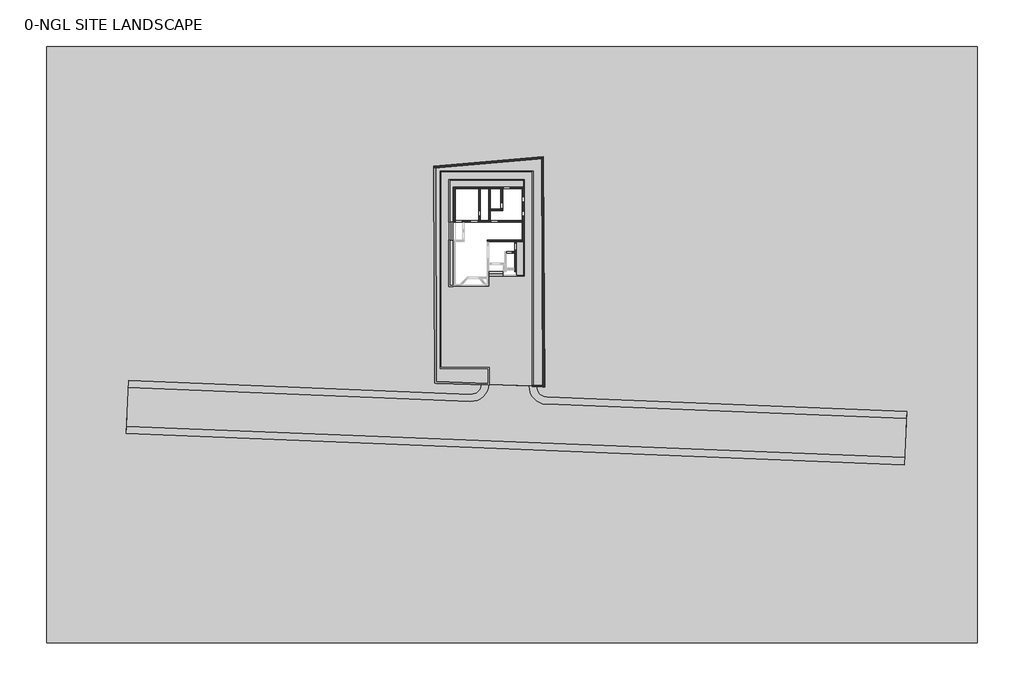
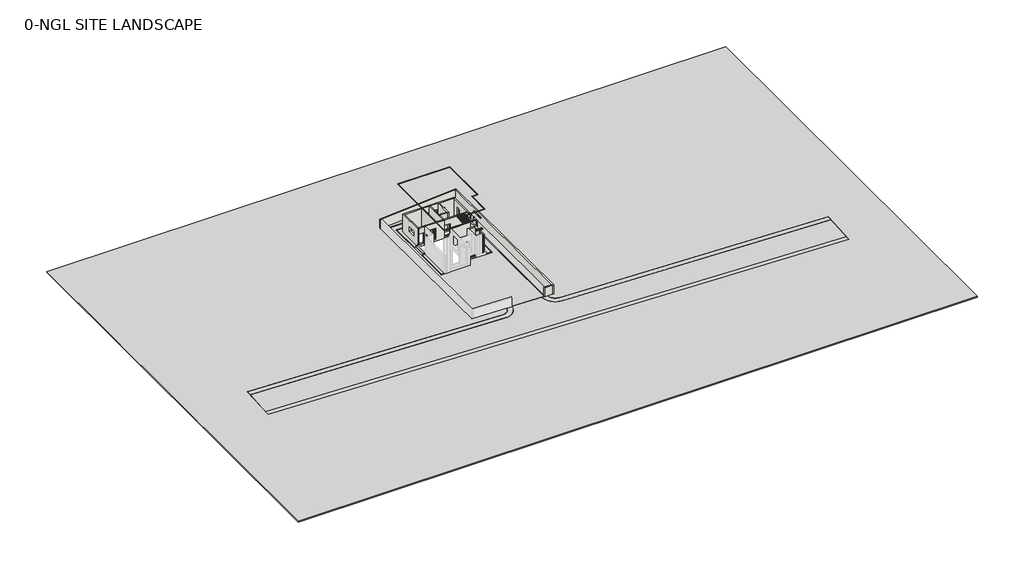
# One storey, part 2 of 2: 21 walls, 2 stair flights, 1 furniture element, 1 proxy.
"""IFC4 building model written with IfcOpenShell, lengths in millimetres."""

from ifc_helpers import new_model, si_unit, frame, origin, origin_with_axes, place, context, project, spatial, polyline, outline, extrude, faceted_brep, transform, mapped, element, save
from components import site_road_site_road_cda8f1bc, casework_1_casework_1_205f5306

model = new_model("IFC4")

# Units and contexts
model_context = context("Model", 3, world=origin())
ifc_project = project(units=[si_unit("LENGTHUNIT", "METRE", prefix="MILLI")], contexts=[model_context])

# Site, building, storey
site = spatial("IfcSite", under=ifc_project)
building = spatial("IfcBuilding", under=site)
storey = spatial("IfcBuildingStorey", under=building, Name="0-NGL SITE LANDSCAPE", Elevation=0.0)

# Proxy
placement = place(None, origin())
site_road_site_road_shape = site_road_site_road_cda8f1bc(model_context)
element("IfcBuildingElementProxy", 1, Name="SITE ROAD : SITE ROAD", ObjectType="SITE ROAD : SITE ROAD", at=placement, inside=storey, context=model_context, shape_type="MappedRepresentation", body=[
    mapped(site_road_site_road_shape, transform((0.0, 0.0, 0.0), x_axis=(1.0, 0.0, 0.0), y_axis=(0.0, 1.0, 0.0), z_axis=(0.0, 0.0, 1.0))),
])

# Furniture
casework_1_casework_1_shape = casework_1_casework_1_205f5306(model_context)
element("IfcFurniture", 2, ObjectType="Casework 1 : Casework 1", at=placement, inside=storey, context=model_context, shape_type="MappedRepresentation", body=[
    mapped(casework_1_casework_1_shape, transform((0.0, 0.0, 0.0), x_axis=(1.0, 0.0, 0.0), y_axis=(0.0, 1.0, 0.0), z_axis=(0.0, 0.0, 1.0))),
])

# Stair flights
element("IfcStairFlight", 3, ObjectType="150mm Depth", at=placement, inside=storey, context=model_context, shape_type="Brep", body=[
    faceted_brep([(-10608.8712297, -1317.0014262, 150.0), (-10908.8712297, -1317.0014262, 150.0), (-10908.8712297, -3817.0014262, 150.0), (-10608.8712297, -3817.0014262, 150.0), (-10608.8712297, -1317.0014262, 0.0), (-10908.8712297, -1317.0014262, 0.0), (-10908.8712297, -3817.0014262, 0.0), (-10608.8712297, -3817.0014262, 0.0), (-10308.8712297, -1317.0014262, 300.0), (-10608.8712297, -1317.0014262, 300.0), (-10608.8712297, -3817.0014262, 300.0), (-10308.8712297, -3817.0014262, 300.0), (-10308.8712297, -1317.0014262, 132.2949017), (-10573.461033, -1317.0014262, 0.0), (-10573.461033, -3817.0014262, 0.0), (-10308.8712297, -3817.0014262, 132.2949017)], [[[0, 1, 2, 3]], [[1, 0, 4, 5]], [[2, 1, 5, 6]], [[3, 2, 6, 7]], [[8, 9, 10, 11]], [[4, 0, 9, 8, 12, 13]], [[0, 3, 10, 9]], [[3, 7, 14, 15, 11, 10]], [[8, 11, 15, 12]], [[5, 4, 13, 14, 7, 6]], [[14, 13, 12, 15]]]),
])
element("IfcStairFlight", 4, ObjectType="150mm Depth", at=placement, inside=storey, context=model_context, shape_type="Brep", body=[
    faceted_brep([(-5348.8712297, -8577.0014262, 150.0), (-5348.8712297, -8877.0014262, 150.0), (-3308.8712297, -8877.0014262, 150.0), (-3308.8712297, -8577.0014262, 150.0), (-5348.8712297, -8577.0014262, 0.0), (-5348.8712297, -8877.0014262, 0.0), (-3308.8712297, -8877.0014262, 0.0), (-3308.8712297, -8577.0014262, 0.0), (-5348.8712297, -8277.0014262, 300.0), (-5348.8712297, -8577.0014262, 300.0), (-3308.8712297, -8577.0014262, 300.0), (-3308.8712297, -8277.0014262, 300.0), (-5348.8712297, -8277.0014262, 132.2949017), (-5348.8712297, -8541.5912295, 0.0), (-3308.8712297, -8541.5912295, 0.0), (-3308.8712297, -8277.0014262, 132.2949017)], [[[0, 1, 2, 3]], [[1, 0, 4, 5]], [[2, 1, 5, 6]], [[3, 2, 6, 7]], [[8, 9, 10, 11]], [[4, 0, 9, 8, 12, 13]], [[0, 3, 10, 9]], [[3, 7, 14, 15, 11, 10]], [[8, 11, 15, 12]], [[5, 4, 13, 14, 7, 6]], [[14, 13, 12, 15]]]),
])

# Walls
element("IfcWall", 5, ObjectType="100", at=placement, inside=storey, context=model_context, shape_type="Brep", body=[
    faceted_brep([(-308.8712297, -8927.0014262, 0.0), (-308.8712297, -4047.0014262, 0.0), (-308.8712297, -4047.0014262, 150.0), (-308.8712297, -8927.0014262, 150.0), (-408.8712297, -8927.0014262, 0.0), (-408.8712297, -8927.0014262, 150.0), (-408.8712297, -8827.0014262, 150.0), (-408.8712297, -4047.0014262, 150.0), (-408.8712297, -4047.0014262, 0.0), (-408.8712297, -8827.0014262, 0.0), (-358.8712297, -4047.0014262, 0.0)], [[[0, 1, 2, 3]], [[4, 5, 6, 7, 8, 9]], [[1, 0, 4, 9, 8, 10]], [[3, 2, 7, 6, 5]], [[2, 1, 10, 8, 7]], [[0, 3, 5, 4]]]),
])
element("IfcWall", 6, ObjectType="100", at=placement, inside=storey, context=model_context, shape_type="Brep", body=[
    faceted_brep([(-10858.8712297, -1317.0014262, 0.0), (-10858.8712297, 4592.9985738, 0.0), (-10858.8712297, 4692.9985738, 0.0), (-10858.8712297, 4692.9985738, 150.0), (-10858.8712297, 4592.9985738, 150.0), (-10858.8712297, -1317.0014262, 150.0), (-10958.8712297, -1317.0014262, 0.0), (-10958.8712297, -1317.0014262, 150.0), (-10958.8712297, 4692.9985738, 150.0), (-10958.8712297, 4692.9985738, 0.0)], [[[0, 1, 2, 3, 4, 5]], [[6, 7, 8, 9]], [[2, 1, 0, 6, 9]], [[5, 4, 3, 8, 7]], [[0, 5, 7, 6]], [[3, 2, 9, 8]]]),
])
element("IfcWall", 7, ObjectType="100", at=placement, inside=storey, context=model_context, shape_type="Brep", body=[
    faceted_brep([(891.1287703, -24267.7575352, 0.0), (891.1287703, 5892.9985738, 0.0), (891.1287703, 5892.9985738, 150.0), (891.1287703, -24267.7575352, 150.0), (791.1287703, -24264.1774027, 0.0), (791.1287703, -24264.1774027, 150.0), (791.1287703, 5792.9985738, 150.0), (791.1287703, 5892.9985738, 150.0), (791.1287703, 5892.9985738, 0.0), (791.1287703, 5792.9985738, 0.0)], [[[0, 1, 2, 3]], [[4, 5, 6, 7, 8, 9]], [[1, 0, 4, 9, 8]], [[3, 2, 7, 6, 5]], [[0, 3, 5, 4]], [[2, 1, 8, 7]]]),
])
element("IfcWall", 8, ObjectType="100", at=placement, inside=storey, context=model_context, shape_type="Brep", body=[
    faceted_brep([(-10858.8712297, 4592.9985738, 0.0), (-408.8712297, 4592.9985738, 0.0), (-308.8712297, 4592.9985738, 0.0), (-308.8712297, 4592.9985738, 150.0), (-408.8712297, 4592.9985738, 150.0), (-10858.8712297, 4592.9985738, 150.0), (-10858.8712297, 4692.9985738, 0.0), (-10858.8712297, 4692.9985738, 150.0), (-308.8712297, 4692.9985738, 150.0), (-308.8712297, 4692.9985738, 0.0)], [[[0, 1, 2, 3, 4, 5]], [[6, 7, 8, 9]], [[2, 1, 0, 6, 9]], [[5, 4, 3, 8, 7]], [[3, 2, 9, 8]], [[0, 5, 7, 6]]]),
])
element("IfcWall", 9, ObjectType="100", at=placement, inside=storey, context=model_context, shape_type="Brep", body=[
    faceted_brep([(-308.8712297, 3642.9985738, 0.0), (-308.8712297, 4592.9985738, 0.0), (-308.8712297, 4592.9985738, 150.0), (-308.8712297, 3642.9985738, 150.0), (-408.8712297, 3642.9985738, 0.0), (-408.8712297, 3642.9985738, 150.0), (-408.8712297, 4592.9985738, 150.0), (-408.8712297, 4592.9985738, 0.0), (-358.8712297, 3642.9985738, 0.0)], [[[0, 1, 2, 3]], [[4, 5, 6, 7]], [[1, 0, 8, 4, 7]], [[3, 2, 6, 5]], [[2, 1, 7, 6]], [[0, 3, 5, 4, 8]]]),
])
element("IfcWall", 10, ObjectType="100", at=placement, inside=storey, context=model_context, shape_type="SweptSolid", body=[
    extrude(outline(polyline([(791.1287703, 5792.9985738), (-12058.8712297, 5792.9985738), (-12058.8712297, 5892.9985738), (791.1287703, 5892.9985738), (791.1287703, 5792.9985738)])), origin_with_axes(), (0.0, 0.0, 1.0), 150.0),
])
element("IfcWall", 11, ObjectType="230", at=placement, inside=storey, context=model_context, shape_type="Brep", body=[
    faceted_brep([(-588.8712297, -3817.0014262, 3750.0), (-588.8712297, -3817.0014262, 0.0), (-5578.8712297, -3817.0014262, 0.0), (-5578.8712297, -3817.0014262, 3750.0), (-588.8712297, -4047.0014262, 0.0), (-588.8712297, -4047.0014262, 3750.0), (-1448.8712297, -4047.0014262, 3750.0), (-1678.8712297, -4047.0014262, 3750.0), (-5348.8712297, -4047.0014262, 3750.0), (-5578.8712297, -4047.0014262, 3750.0), (-5578.8712297, -4047.0014262, 0.0), (-5348.8712297, -4047.0014262, 0.0), (-1678.8712297, -4047.0014262, 0.0), (-1448.8712297, -4047.0014262, 0.0)], [[[0, 1, 2, 3]], [[4, 5, 6, 7, 8, 9, 10, 11, 12, 13]], [[2, 1, 4, 13, 12, 11, 10]], [[0, 3, 9, 8, 7, 6, 5]], [[3, 2, 10, 9]], [[0, 5, 4, 1]]]),
])
element("IfcWall", 12, ObjectType="230", at=placement, inside=storey, context=model_context, shape_type="Brep", body=[
    faceted_brep([(-10308.8712297, 3642.9985738, 0.0), (-10308.8712297, -1202.0014262, 0.0), (-10308.8712297, -1202.0014262, 450.0), (-10308.8712297, -1317.0014262, 450.0), (-10308.8712297, -1317.0014262, 3750.0), (-10308.8712297, 3642.9985738, 3750.0), (-10308.8712297, -82.0014262, 1650.0), (-10308.8712297, 1417.9985738, 1650.0), (-10308.8712297, 1417.9985738, 2550.0), (-10308.8712297, -82.0014262, 2550.0), (-10078.8712297, 3642.9985738, 0.0), (-10078.8712297, 3642.9985738, 3750.0), (-10078.8712297, 3412.9985738, 3750.0), (-10078.8712297, -1087.0014262, 3750.0), (-10078.8712297, -1317.0014262, 3750.0), (-10078.8712297, -1317.0014262, 450.0), (-10078.8712297, -1202.0014262, 450.0), (-10078.8712297, -1202.0014262, 0.0), (-10078.8712297, -1087.0014262, 0.0), (-10078.8712297, 3412.9985738, 0.0), (-10078.8712297, -82.0014262, 1650.0), (-10078.8712297, -82.0014262, 2550.0), (-10078.8712297, 1417.9985738, 2550.0), (-10078.8712297, 1417.9985738, 1650.0)], [[[0, 1, 2, 3, 4, 5], [6, 7, 8, 9]], [[10, 11, 12, 13, 14, 15, 16, 17, 18, 19], [20, 21, 22, 23]], [[1, 0, 10, 19, 18, 17]], [[5, 4, 14, 13, 12, 11]], [[0, 5, 11, 10]], [[21, 20, 6, 9]], [[22, 21, 9, 8]], [[23, 22, 8, 7]], [[20, 23, 7, 6]], [[2, 1, 17, 16]], [[15, 3, 2, 16]], [[4, 3, 15, 14]]]),
])
element("IfcWall", 13, ObjectType="230", at=placement, inside=storey, context=model_context, shape_type="Brep", body=[
    faceted_brep([(-1448.8712297, -8277.0014262, 0.0), (-1448.8712297, -4047.0014262, 0.0), (-1448.8712297, -4047.0014262, 3750.0), (-1448.8712297, -8277.0014262, 3750.0), (-1448.8712297, -8277.0014262, 500.0), (-1448.8712297, -4239.5014262, 900.0), (-1448.8712297, -5239.5014262, 900.0), (-1448.8712297, -5239.5014262, 2550.0), (-1448.8712297, -4239.5014262, 2550.0), (-1448.8712297, -6482.0014262, 1950.0), (-1448.8712297, -7382.0014262, 1950.0), (-1448.8712297, -7382.0014262, 2550.0), (-1448.8712297, -6482.0014262, 2550.0), (-1678.8712297, -8277.0014262, 0.0), (-1678.8712297, -8277.0014262, 3750.0), (-1678.8712297, -8047.0014262, 3750.0), (-1678.8712297, -7817.0014262, 3750.0), (-1678.8712297, -5662.0014262, 3750.0), (-1678.8712297, -5432.0014262, 3750.0), (-1678.8712297, -4047.0014262, 3750.0), (-1678.8712297, -4047.0014262, 0.0), (-1678.8712297, -5432.0014262, 0.0), (-1678.8712297, -5662.0014262, 0.0), (-1678.8712297, -7817.0014262, 0.0), (-1678.8712297, -8047.0014262, 0.0), (-1678.8712297, -4239.5014262, 900.0), (-1678.8712297, -4239.5014262, 2550.0), (-1678.8712297, -5239.5014262, 2550.0), (-1678.8712297, -5239.5014262, 900.0), (-1678.8712297, -6482.0014262, 1950.0), (-1678.8712297, -6482.0014262, 2550.0), (-1678.8712297, -7382.0014262, 2550.0), (-1678.8712297, -7382.0014262, 1950.0), (-1548.8712297, -8277.0014262, 0.0)], [[[0, 1, 2, 3, 4], [5, 6, 7, 8], [9, 10, 11, 12]], [[13, 14, 15, 16, 17, 18, 19, 20, 21, 22, 23, 24], [25, 26, 27, 28], [29, 30, 31, 32]], [[1, 0, 33, 13, 24, 23, 22, 21, 20]], [[3, 2, 19, 18, 17, 16, 15, 14]], [[0, 4, 3, 14, 13, 33]], [[2, 1, 20, 19]], [[26, 25, 5, 8]], [[27, 26, 8, 7]], [[28, 27, 7, 6]], [[25, 28, 6, 5]], [[30, 29, 9, 12]], [[31, 30, 12, 11]], [[32, 31, 11, 10]], [[29, 32, 10, 9]]]),
])
element("IfcWall", 14, ObjectType="230", at=placement, inside=storey, context=model_context, shape_type="Brep", body=[
    faceted_brep([(-10078.8712297, -1317.0014262, 0.0), (-9008.8712297, -1317.0014262, 0.0), (-8778.8712297, -1317.0014262, 0.0), (-5118.8712297, -1317.0014262, 0.0), (-5118.8712297, -1317.0014262, 3750.0), (-8778.8712297, -1317.0014262, 3750.0), (-9008.8712297, -1317.0014262, 3750.0), (-10078.8712297, -1317.0014262, 3750.0), (-10078.8712297, -1317.0014262, 450.0), (-9068.8712297, -1317.0014262, 450.0), (-10018.8712297, -1317.0014262, 450.0), (-10018.8712297, -1317.0014262, 2575.0), (-9068.8712297, -1317.0014262, 2575.0), (-7916.1212297, -1317.0014262, 2639.5), (-6811.6212297, -1317.0014262, 2639.5), (-6811.6212297, -1317.0014262, 450.0), (-7916.1212297, -1317.0014262, 450.0), (-5118.8712297, -1087.0014262, 0.0), (-5348.8712297, -1087.0014262, 0.0), (-6548.8712297, -1087.0014262, 0.0), (-6778.8712297, -1087.0014262, 0.0), (-10078.8712297, -1087.0014262, 0.0), (-10078.8712297, -1087.0014262, 3750.0), (-6778.8712297, -1087.0014262, 3750.0), (-6548.8712297, -1087.0014262, 3750.0), (-5348.8712297, -1087.0014262, 3750.0), (-5118.8712297, -1087.0014262, 3750.0), (-9068.8712297, -1087.0014262, 450.0), (-9068.8712297, -1087.0014262, 2575.0), (-10018.8712297, -1087.0014262, 2575.0), (-10018.8712297, -1087.0014262, 450.0), (-6811.6212297, -1087.0014262, 2639.5), (-7916.1212297, -1087.0014262, 2639.5), (-7916.1212297, -1087.0014262, 450.0), (-6811.6212297, -1087.0014262, 450.0), (-10078.8712297, -1202.0014262, 0.0), (-6811.6212297, -1107.0014262, 2639.5), (-7916.1212297, -1107.0014262, 2639.5), (-7916.1212297, -1184.0014262, 2639.5), (-6811.6212297, -1184.0014262, 2639.5), (-6811.6212297, -1107.0014262, 450.0), (-6811.6212297, -1184.0014262, 450.0), (-7916.1212297, -1107.0014262, 450.0), (-7931.1212297, -1107.0014262, 450.0), (-7931.1212297, -1184.0014262, 450.0), (-7916.1212297, -1184.0014262, 450.0), (-6796.6212297, -1184.0014262, 450.0), (-6796.6212297, -1107.0014262, 450.0), (-7931.1212297, -1107.0014262, 2654.5), (-6796.6212297, -1107.0014262, 2654.5), (-6796.6212297, -1184.0014262, 2654.5), (-7931.1212297, -1184.0014262, 2654.5)], [[[0, 1, 2, 3, 4, 5, 6, 7, 8], [9, 10, 11, 12], [13, 14, 15, 16]], [[17, 18, 19, 20, 21, 22, 23, 24, 25, 26], [27, 28, 29, 30], [31, 32, 33, 34]], [[3, 2, 1, 0, 35, 21, 20, 19, 18, 17]], [[7, 6, 5, 4, 26, 25, 24, 23, 22]], [[4, 3, 17, 26]], [[7, 22, 21, 35, 0, 8]], [[28, 27, 9, 12]], [[29, 28, 12, 11]], [[30, 29, 11, 10]], [[27, 30, 10, 9]], [[31, 36, 37, 32]], [[13, 38, 39, 14]], [[36, 31, 34, 40]], [[14, 39, 41, 15]], [[40, 34, 33, 42, 43, 44, 45, 16, 15, 41, 46, 47]], [[32, 37, 42, 33]], [[38, 13, 16, 45]], [[48, 49, 50, 51]], [[47, 46, 50, 49]], [[39, 38, 45, 44, 51, 50, 46, 41]], [[44, 43, 48, 51]], [[37, 36, 40, 47, 49, 48, 43, 42]]]),
])
element("IfcWall", 15, ObjectType="230", at=placement, inside=storey, context=model_context, shape_type="Brep", body=[
    faceted_brep([(-5348.8712297, 3412.9985738, 0.0), (-5348.8712297, -1087.0014262, 0.0), (-5348.8712297, -1087.0014262, 3750.0), (-5348.8712297, 3412.9985738, 3750.0), (-5118.8712297, 3412.9985738, 0.0), (-5118.8712297, 3412.9985738, 3750.0), (-5118.8712297, 512.9985738, 3750.0), (-5118.8712297, 282.9985738, 3750.0), (-5118.8712297, -1087.0014262, 3750.0), (-5118.8712297, -1087.0014262, 0.0), (-5118.8712297, 282.9985738, 0.0), (-5118.8712297, 512.9985738, 0.0)], [[[0, 1, 2, 3]], [[4, 5, 6, 7, 8, 9, 10, 11]], [[1, 0, 4, 11, 10, 9]], [[3, 2, 8, 7, 6, 5]], [[0, 3, 5, 4]], [[2, 1, 9, 8]]]),
])
element("IfcWall", 16, ObjectType="230", at=placement, inside=storey, context=model_context, shape_type="Brep", body=[
    faceted_brep([(-10078.8712297, 3412.9985738, 0.0), (-6778.8712297, 3412.9985738, 0.0), (-6548.8712297, 3412.9985738, 0.0), (-5348.8712297, 3412.9985738, 0.0), (-5118.8712297, 3412.9985738, 0.0), (-3618.8712297, 3412.9985738, 0.0), (-3388.8712297, 3412.9985738, 0.0), (-588.8712297, 3412.9985738, 0.0), (-358.8712297, 3412.9985738, 0.0), (-358.8712297, 3412.9985738, 3750.0), (-588.8712297, 3412.9985738, 3750.0), (-3388.8712297, 3412.9985738, 3750.0), (-3618.8712297, 3412.9985738, 3750.0), (-5118.8712297, 3412.9985738, 3750.0), (-5348.8712297, 3412.9985738, 3750.0), (-6548.8712297, 3412.9985738, 3750.0), (-6778.8712297, 3412.9985738, 3750.0), (-10078.8712297, 3412.9985738, 3750.0), (-3303.8712297, 3412.9985738, 900.0), (-3303.8712297, 3412.9985738, 2550.0), (-2303.8712297, 3412.9985738, 2550.0), (-2303.8712297, 3412.9985738, 900.0), (-6398.8712297, 3412.9985738, 1950.0), (-6398.8712297, 3412.9985738, 2550.0), (-5498.8712297, 3412.9985738, 2550.0), (-5498.8712297, 3412.9985738, 1950.0), (-4818.8712297, 3412.9985738, 1950.0), (-4818.8712297, 3412.9985738, 2550.0), (-3918.8712297, 3412.9985738, 2550.0), (-3918.8712297, 3412.9985738, 1950.0), (-10078.8712297, 3642.9985738, 0.0), (-10078.8712297, 3642.9985738, 3750.0), (-358.8712297, 3642.9985738, 3750.0), (-358.8712297, 3642.9985738, 0.0), (-408.8712297, 3642.9985738, 0.0), (-3303.8712297, 3642.9985738, 900.0), (-2303.8712297, 3642.9985738, 900.0), (-2303.8712297, 3642.9985738, 2550.0), (-3303.8712297, 3642.9985738, 2550.0), (-6398.8712297, 3642.9985738, 1950.0), (-5498.8712297, 3642.9985738, 1950.0), (-5498.8712297, 3642.9985738, 2550.0), (-6398.8712297, 3642.9985738, 2550.0), (-4818.8712297, 3642.9985738, 1950.0), (-3918.8712297, 3642.9985738, 1950.0), (-3918.8712297, 3642.9985738, 2550.0), (-4818.8712297, 3642.9985738, 2550.0)], [[[0, 1, 2, 3, 4, 5, 6, 7, 8, 9, 10, 11, 12, 13, 14, 15, 16, 17], [18, 19, 20, 21], [22, 23, 24, 25], [26, 27, 28, 29]], [[30, 31, 32, 33, 34], [35, 36, 37, 38], [39, 40, 41, 42], [43, 44, 45, 46]], [[8, 7, 6, 5, 4, 3, 2, 1, 0, 30, 34, 33]], [[17, 16, 15, 14, 13, 12, 11, 10, 9, 32, 31]], [[0, 17, 31, 30]], [[19, 18, 35, 38]], [[20, 19, 38, 37]], [[21, 20, 37, 36]], [[18, 21, 36, 35]], [[23, 22, 39, 42]], [[24, 23, 42, 41]], [[25, 24, 41, 40]], [[22, 25, 40, 39]], [[27, 26, 43, 46]], [[28, 27, 46, 45]], [[29, 28, 45, 44]], [[26, 29, 44, 43]], [[8, 33, 32, 9]]]),
])
element("IfcWall", 17, ObjectType="230", at=placement, inside=storey, context=model_context, shape_type="SweptSolid", body=[
    extrude(outline(polyline([(3412.9985738, 0.0), (-1087.0014262, 0.0), (-1087.0014262, 3750.0), (3412.9985738, 3750.0), (3412.9985738, 0.0)]), holes=[polyline([(-502.0014262, 450.0), (297.9985738, 450.0), (297.9985738, 2575.0), (-502.0014262, 2575.0), (-502.0014262, 450.0)])]), frame((-6778.8712297, 0.0, 0.0), z_axis=(1.0, 0.0, 0.0), x_axis=(0.0, 1.0, 0.0)), (0.0, 0.0, 1.0), 230.0),
])
element("IfcWall", 18, ObjectType="230", at=placement, inside=storey, context=model_context, shape_type="Brep", body=[
    faceted_brep([(-3618.8712297, 3412.9985738, 0.0), (-3618.8712297, 512.9985738, 0.0), (-3618.8712297, 282.9985738, 0.0), (-3618.8712297, 282.9985738, 3750.0), (-3618.8712297, 512.9985738, 3750.0), (-3618.8712297, 3412.9985738, 3750.0), (-3618.8712297, 597.9985738, 450.0), (-3618.8712297, 1397.9985738, 450.0), (-3618.8712297, 1397.9985738, 2575.0), (-3618.8712297, 597.9985738, 2575.0), (-3388.8712297, 3412.9985738, 0.0), (-3388.8712297, 3412.9985738, 3750.0), (-3388.8712297, 282.9985738, 3750.0), (-3388.8712297, 282.9985738, 0.0), (-3388.8712297, 597.9985738, 450.0), (-3388.8712297, 597.9985738, 2575.0), (-3388.8712297, 1397.9985738, 2575.0), (-3388.8712297, 1397.9985738, 450.0)], [[[0, 1, 2, 3, 4, 5], [6, 7, 8, 9]], [[10, 11, 12, 13], [14, 15, 16, 17]], [[2, 1, 0, 10, 13]], [[5, 4, 3, 12, 11]], [[0, 5, 11, 10]], [[3, 2, 13, 12]], [[15, 14, 6, 9]], [[16, 15, 9, 8]], [[17, 16, 8, 7]], [[14, 17, 7, 6]]]),
])
element("IfcWall", 19, ObjectType="230", at=placement, inside=storey, context=model_context, shape_type="SweptSolid", body=[
    extrude(outline(polyline([(-5118.8712297, 512.9985738), (-3618.8712297, 512.9985738), (-3618.8712297, 282.9985738), (-5118.8712297, 282.9985738), (-5118.8712297, 512.9985738)])), origin_with_axes(), (0.0, 0.0, 1.0), 3750.0),
])
element("IfcWall", 20, ObjectType="230", at=placement, inside=storey, context=model_context, shape_type="Brep", body=[
    faceted_brep([(-588.8712297, 3412.9985738, 0.0), (-588.8712297, -1087.0014262, 0.0), (-588.8712297, -1317.0014262, 0.0), (-588.8712297, -3817.0014262, 0.0), (-588.8712297, -4047.0014262, 0.0), (-588.8712297, -4047.0014262, 3750.0), (-588.8712297, -3817.0014262, 3750.0), (-588.8712297, -3080.571442, 3750.0), (-588.8712297, -3080.571442, 1950.0), (-588.8712297, -1880.571442, 1950.0), (-588.8712297, -1880.571442, 3750.0), (-588.8712297, -1317.0014262, 3750.0), (-588.8712297, -1087.0014262, 3750.0), (-588.8712297, 3412.9985738, 3750.0), (-588.8712297, 2272.9985738, 900.0), (-588.8712297, 2272.9985738, 2550.0), (-588.8712297, 1522.9985738, 2550.0), (-588.8712297, 1522.9985738, 900.0), (-588.8712297, 262.9985738, 900.0), (-588.8712297, 262.9985738, 2550.0), (-588.8712297, -487.0014262, 2550.0), (-588.8712297, -487.0014262, 900.0), (-358.8712297, -4047.0014262, 0.0), (-358.8712297, 3412.9985738, 0.0), (-358.8712297, 3412.9985738, 3750.0), (-358.8712297, -1880.571442, 3750.0), (-358.8712297, -1880.571442, 1950.0), (-358.8712297, -3080.571442, 1950.0), (-358.8712297, -3080.571442, 3750.0), (-358.8712297, -4047.0014262, 3750.0), (-358.8712297, 2272.9985738, 900.0), (-358.8712297, 1522.9985738, 900.0), (-358.8712297, 1522.9985738, 2550.0), (-358.8712297, 2272.9985738, 2550.0), (-358.8712297, 262.9985738, 900.0), (-358.8712297, -487.0014262, 900.0), (-358.8712297, -487.0014262, 2550.0), (-358.8712297, 262.9985738, 2550.0), (-408.8712297, -4047.0014262, 0.0)], [[[0, 1, 2, 3, 4, 5, 6, 7, 8, 9, 10, 11, 12, 13], [14, 15, 16, 17], [18, 19, 20, 21]], [[22, 23, 24, 25, 26, 27, 28, 29], [30, 31, 32, 33], [34, 35, 36, 37]], [[4, 3, 2, 1, 0, 23, 22, 38]], [[24, 13, 12, 11, 10, 25]], [[5, 29, 28, 7, 6]], [[15, 14, 30, 33]], [[16, 15, 33, 32]], [[17, 16, 32, 31]], [[14, 17, 31, 30]], [[19, 18, 34, 37]], [[20, 19, 37, 36]], [[21, 20, 36, 35]], [[18, 21, 35, 34]], [[9, 26, 25, 10]], [[27, 8, 7, 28]], [[26, 9, 8, 27]], [[4, 38, 22, 29, 5]], [[13, 24, 23, 0]]]),
])
element("IfcWall", 21, ObjectType="230", at=placement, inside=storey, context=model_context, shape_type="Brep", body=[
    faceted_brep([(-5118.8712297, -1317.0014262, 0.0), (-588.8712297, -1317.0014262, 0.0), (-588.8712297, -1317.0014262, 3750.0), (-5118.8712297, -1317.0014262, 3750.0), (-5086.1212297, -1317.0014262, 2639.5), (-3981.6212297, -1317.0014262, 2639.5), (-3981.6212297, -1317.0014262, 450.0), (-5086.1212297, -1317.0014262, 450.0), (-588.8712297, -1087.0014262, 0.0), (-5118.8712297, -1087.0014262, 0.0), (-5118.8712297, -1087.0014262, 3750.0), (-588.8712297, -1087.0014262, 3750.0), (-3981.6212297, -1087.0014262, 2639.5), (-5086.1212297, -1087.0014262, 2639.5), (-5086.1212297, -1087.0014262, 450.0), (-3981.6212297, -1087.0014262, 450.0), (-3981.6212297, -1107.0014262, 2639.5), (-5086.1212297, -1107.0014262, 2639.5), (-5086.1212297, -1184.0014262, 2639.5), (-3981.6212297, -1184.0014262, 2639.5), (-5086.1212297, -1107.0014262, 450.0), (-5086.1212297, -1184.0014262, 450.0), (-5101.1212297, -1107.0014262, 450.0), (-5101.1212297, -1184.0014262, 450.0), (-3981.6212297, -1184.0014262, 450.0), (-3966.6212297, -1184.0014262, 450.0), (-3966.6212297, -1107.0014262, 450.0), (-3981.6212297, -1107.0014262, 450.0), (-3966.6212297, -1107.0014262, 2654.5), (-3966.6212297, -1184.0014262, 2654.5), (-5101.1212297, -1184.0014262, 2654.5), (-5101.1212297, -1107.0014262, 2654.5)], [[[0, 1, 2, 3], [4, 5, 6, 7]], [[8, 9, 10, 11], [12, 13, 14, 15]], [[1, 0, 9, 8]], [[3, 2, 11, 10]], [[0, 3, 10, 9]], [[2, 1, 8, 11]], [[12, 16, 17, 13]], [[4, 18, 19, 5]], [[13, 17, 20, 14]], [[18, 4, 7, 21]], [[14, 20, 22, 23, 21, 7, 6, 24, 25, 26, 27, 15]], [[16, 12, 15, 27]], [[5, 19, 24, 6]], [[28, 29, 30, 31]], [[23, 22, 31, 30]], [[19, 18, 21, 23, 30, 29, 25, 24]], [[26, 25, 29, 28]], [[17, 16, 27, 26, 28, 31, 22, 20]]]),
])
element("IfcWall", 22, ObjectType="230", at=placement, inside=storey, context=model_context, shape_type="SweptSolid", body=[
    extrude(outline(polyline([(0.0, -2848.8712297), (0.0, -1678.8712297), (3750.0, -1678.8712297), (3750.0, -2848.8712297), (2575.0, -2848.8712297), (2575.0, -2063.8712297), (450.0, -2063.8712297), (450.0, -2848.8712297), (0.0, -2848.8712297)])), frame((0.0, -5662.0014262, 0.0), z_axis=(0.0, 1.0, 0.0), x_axis=(0.0, 0.0, 1.0)), (0.0, 0.0, 1.0), 230.0),
])
element("IfcWall", 23, ObjectType="230", at=placement, inside=storey, context=model_context, shape_type="Brep", body=[
    faceted_brep([(-13056.2467144, 6312.39333, 0.0), (-12826.325768, 6332.305069, 0.0), (2127.0679152, 7627.3070062, 0.0), (2356.9669464, 7647.2168472, 0.0), (2356.9669464, 7647.2168472, 1950.0), (2127.0679152, 7627.3070062, 1950.0), (-12826.325768, 6332.305069, 1950.0), (-13056.2467144, 6312.39333, 1950.0), (-13057.1849874, 6543.1729621, 0.0), (-13057.1849874, 6543.1729621, 1950.0), (2355.7602649, 7877.9732344, 1950.0), (2355.7602649, 7877.9732344, 0.0)], [[[0, 1, 2, 3, 4, 5, 6, 7]], [[8, 9, 10, 11]], [[3, 2, 1, 0, 8, 11]], [[7, 6, 5, 4, 10, 9]], [[4, 3, 11, 10]], [[0, 7, 9, 8]]]),
])
element("IfcWall", 24, ObjectType="230", at=placement, inside=storey, context=model_context, shape_type="Brep", body=[
    faceted_brep([(2127.0679152, 7627.3070062, 0.0), (2294.11766, -24317.9863963, 0.0), (2295.3213821, -24548.1768434, 0.0), (2295.3213821, -24548.1768434, 1950.0), (2294.11766, -24317.9863963, 1950.0), (2127.0679152, 7627.3070062, 1950.0), (2356.9669464, 7647.2168472, 0.0), (2356.9669464, 7647.2168472, 1950.0), (2525.3675946, -24556.4128027, 1950.0), (2525.3675946, -24556.4128027, 0.0)], [[[0, 1, 2, 3, 4, 5]], [[6, 7, 8, 9]], [[2, 1, 0, 6, 9]], [[5, 4, 3, 8, 7]], [[0, 5, 7, 6]], [[3, 2, 9, 8]]]),
])
element("IfcWall", 25, ObjectType="230", at=placement, inside=storey, context=model_context, shape_type="Brep", body=[
    faceted_brep([(791.1287703, -24494.324755, 0.0), (2295.3213821, -24548.1768434, 0.0), (2295.3213821, -24548.1768434, 1950.0), (791.1287703, -24494.324755, 1950.0), (791.1287703, -24264.1774027, 0.0), (791.1287703, -24264.1774027, 150.0), (791.1287703, -24264.1774027, 1950.0), (2294.11766, -24317.9863963, 1950.0), (2294.11766, -24317.9863963, 0.0), (891.1287703, -24267.7575352, 0.0)], [[[0, 1, 2, 3]], [[4, 5, 6, 7, 8, 9]], [[1, 0, 4, 9, 8]], [[3, 2, 7, 6]], [[2, 1, 8, 7]], [[0, 3, 6, 5, 4]]]),
])

save(model, "model.ifc")

# Revit data of these elements
# Type "100"
#   Layers, outside or top first: 100 mm "Default Wall" (function 1)
# Type "230"
#   Layers, outside or top first: 230 mm "Default Wall" (function 1)
# Element 1 (IfcBuildingElementProxy, "SITE ROAD : SITE ROAD")
#   Phase Created = New Construction
#   Materials on its faces: "Grass 02", "Pavement 13, Herringbone", "Concrete 04"
# Element 2 (IfcFurniture, "Casework 1 : Casework 1")
#   Phase Created = New Construction
#   Materials on its faces: "Iron, Ductile", "J LIGHT", "J POP"
# Elements 3, 4 (IfcStairFlight, "150mm Depth")
#   Phase Created = New Construction
#   Materials on its faces: "Marble 06"
# Elements 5, 6, 7, 8, 9, 10 (IfcWall, "100")
#   Top Offset = 150 mm
#   Base Offset = 0 mm
#   wall height = 150 mm
#   Phase Created = New Construction
#   Base Constraint = 0-NGL SITE LANDSCAPE
#   Top Constraint = 0-NGL SITE LANDSCAPE
#   Materials on its faces: "Default Wall"
# Elements 11, 12, 13, 14, 15, 16, 17, 18, 19, 20, 21, 22 (IfcWall, "230")
#   Top Offset = 0 mm
#   Base Offset = 0 mm
#   wall height = 3750 mm
#   Phase Created = New Construction
#   Base Constraint = 0-NGL SITE LANDSCAPE
#   Top Constraint = S1
#   Materials on its faces: "Default Wall"
# Elements 23, 24, 25 (IfcWall, "230")
#   Top Offset = 1500 mm
#   Base Offset = 0 mm
#   wall height = 1950 mm
#   Phase Created = New Construction
#   Base Constraint = 0-NGL SITE LANDSCAPE
#   Top Constraint = 01- GROUND FLOOR
#   Materials on its faces: "Default Wall"
# Materials
#   "Default Wall": colour RGB 255 255 255, transparency 0, Cost = 0
#   "Grass 02": colour RGB 100 122 63, transparency 0, Cost = 0
#   "Pavement 13, Herringbone": colour RGB 134 134 134, transparency 0, Cost = 0
#   "Concrete 04": colour RGB 80 80 80, transparency 0
#   "Iron, Ductile": class "Metal", colour RGB 90 97 102, transparency 0, Description = "Ductile cast iron", Cost = 0
#   "J LIGHT": class "Generic", colour RGB 255 255 0, transparency 0, Cost = 0
#   "J POP": class "Generic", colour RGB 255 255 255, transparency 0, Cost = 0
#   "Marble 06": colour RGB 58 58 58, transparency 0, Cost = 0
